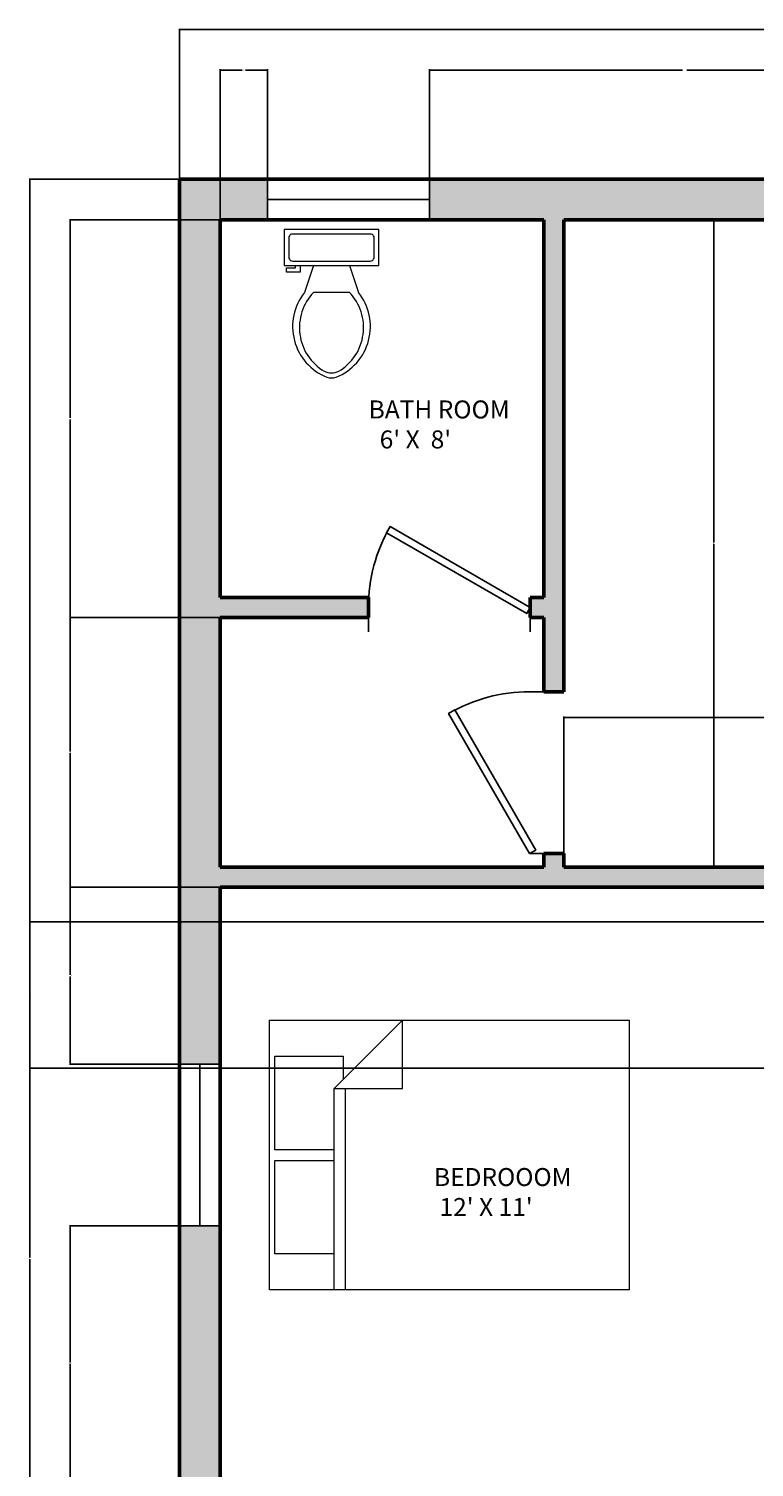
# Model space of a CAD drawing. Units: inches. Extents: x 4 to 671, y -79 to 570.
# Tile 3 of 7: x 4 to 165, y 250 to 570. Entities that reach past the tile are written whole.
import ezdxf

# ---------------------------------------------------------------- set-up
doc = ezdxf.new("R2010")
doc.units = ezdxf.units.IN
doc.header["$MEASUREMENT"] = 0
for name, color, linetype, lineweight in [('A-ANNO-DIMS', 2, 'Continuous', 18), ('A-AREA-IDEN', 7, 'Continuous', 18), ('A-WALL', 7, 'Continuous', 50), ('A-WALL-PATT', 251, 'Continuous', 13), ('bathroom', 90, 'Continuous', 18), ('doors', 40, 'Continuous', 25), ('furniture', 220, 'Continuous', 18), ('window', 30, 'Continuous', 25)]:
    doc.layers.add(name, color=color, linetype=linetype, lineweight=lineweight)
doc.styles.get("Standard").update_dxf_attribs({"font": 'arial.ttf'})
doc.dimstyles.get("Standard").update_dxf_attribs({"dimtxt": 0.18, "dimasz": 0.18, "dimexe": 0.18, "dimexo": 0.0625, "dimgap": 0.09, "dimtad": 0, "dimtih": 1, "dimtoh": 1, "dimdec": 4, "dimzin": 0, "dimdsep": 46, "dimtxsty": 'Standard', "dimcen": 0.09, "dimadec": 0, "dimazin": 0, "dimtfac": 1, "dimtdec": 4, "dimtofl": 0, "dimtmove": 0, "dimatfit": 3, "dimfxl": 1, "dimtolj": 1, "dimtzin": 0, "dimarcsym": 0})

# ---------------------------------------------------------------- blocks, each defined once
blk = doc.blocks.new('*U9')
for p, q in [((0, 0), (0, -6)), ((40, 0), (40, -6))]:
    blk.add_line(p, q)
blk.add_lwpolyline([(0, 0), (34.64, 20), (35.52, 18.48), (0.87, -1.52)], close=True)
blk.add_arc((0, 0), 40, 0, 30)
blk = doc.blocks.new('*U11')
for p, q in [((0, 0), (0, 6)), ((40, 0), (40, 6))]:
    blk.add_line(p, q)
blk.add_lwpolyline([(0, 0), (34.64, -20), (35.52, -18.48), (0.87, 1.52)], close=True)
blk.add_arc((0, 0), 40, 330, 0)
blk = doc.blocks.new('Bed - Queen')
for p, q in [((0, -80.00003), (0, 0)), ((0, 0), (59.99999, 0)), ((59.99999, 0), (59.99999, -80.00003)), ((7.99999, -1.2), (28.79998, -1.2)), ((7.99999, -14.4), (7.99999, -1.2)), ((28.79998, -1.2), (28.79998, -14.4)), ((31.19999, -1.2), (51.99999, -1.2)), ((31.19999, -14.4), (31.19999, -1.2)), ((51.99999, -1.2), (51.99999, -16.4)), ((0, -14.4), (44.8, -14.4)), ((59.99999, -29.6), (44.8, -14.4)), ((44.8, -14.4), (44.8, -29.6)), ((44.8, -16.8), (0, -16.8)), ((51.99999, -16.4), (46.79936, -16.4)), ((44.8, -29.6), (59.99999, -29.6)), ((59.99999, -80.00003), (0, -80.00003))]:
    blk.add_line(p, q)
blk = doc.blocks.new('Toilet - top')
for p, q in [((9.5, -6), (9.5, -2)), ((-10, -8.5), (-8, -8.5)), ((-10, -9.5), (-10, -8.5)), ((-7, -9.5), (-10, -9.5)), ((-8, -8.5), (-8, -8)), ((-7, -8), (-7, -9.5)), ((-4, -8), (-6, -14)), ((4, -8), (6, -14)), ((4, -14), (-4, -14))]:
    blk.add_line(p, q)
blk.add_lwpolyline([(10.5, -8), (10.5, 0), (-10.5, 0), (-10.5, -8)], close=True)
for points in [[(-9.5, -2), (-9.5, -6)], [(8.5, -1), (-8.5, -1)], [(-8.5, -7), (8.5, -7)]]:
    blk.add_lwpolyline(points)
for centre, radius, start, end in [((-8.62, -1.88), 0.884, 81.8699, 188.1301), ((8.62, -1.88), 0.884, 351.8699, 98.1301), ((-8.62, -6.12), 0.884, 171.8699, 278.1301), ((8.62, -6.12), 0.884, 261.8699, 8.1301), ((3.52, -21.58), 12.17, 141.4691, 247.9714), ((4.2, -21.82), 11.33, 136.3677, 238.9468), ((-3.52, -21.58), 12.17, 292.0284, 38.5307), ((-4.2, -21.82), 11.33, 301.053, 43.6321), ((0, -27.88), 4, 245.7318, 294.2682), ((0, -29), 4, 254.8605, 285.1395)]:
    blk.add_arc(centre, radius, start, end)
blk = doc.blocks.new('WIN-36')
for p, q in [((0, 0), (0, 9)), ((0, 9), (36, 9)), ((36, 9), (36, 0)), ((36, 9), (36, 4.5)), ((36, 4.5), (0, 4.5)), ((36, 0), (0, 0))]:
    blk.add_line(p, q)
blk = doc.blocks.new('*D49')
at = {"layer": 'A-ANNO-DIMS', "color": 0, "lineweight": -2, "transparency": 16777216}
for p, q in [((37.44, 536.41), (37.44, 569.83)), ((37.62, 569.65), (337.15, 569.65)), ((637.26, 569.65), (337.73, 569.65)), ((637.44, 536.41), (637.44, 569.83))]:
    blk.add_line(p, q, dxfattribs=at)
at = {"layer": 'A-ANNO-DIMS', "color": 0, "transparency": 16777216}
for points in [[(37.62, 569.68), (37.62, 569.62), (37.44, 569.65)], [(637.26, 569.68), (637.26, 569.62), (637.44, 569.65)]]:
    blk.add_solid(points, dxfattribs=at)
at = {"layer": 'Defpoints', "color": 0, "transparency": 16777216}
for p in [(637.44, 569.65), (37.44, 536.35), (637.44, 536.35)]:
    blk.add_point(p, dxfattribs=at)
at = {"layer": 'A-ANNO-DIMS', "color": 0, "transparency": 16777216, "insert": (337.44, 569.65), "char_height": 0.18, "attachment_point": 5}
blk.add_mtext('\\A1;600', dxfattribs=at)
blk = doc.blocks.new('*D51')
at = {"layer": 'A-ANNO-DIMS', "color": 0, "lineweight": -2, "transparency": 16777216}
for p, q in [((37.38, 536.35), (3.96, 536.35)), ((4.14, 536.17), (4.14, 296.53)), ((4.14, 56.53), (4.14, 296.17)), ((37.38, 56.35), (3.96, 56.35))]:
    blk.add_line(p, q, dxfattribs=at)
at = {"layer": 'A-ANNO-DIMS', "color": 0, "transparency": 16777216}
for points in [[(4.11, 536.17), (4.17, 536.17), (4.14, 536.35)], [(4.11, 56.53), (4.17, 56.53), (4.14, 56.35)]]:
    blk.add_solid(points, dxfattribs=at)
at = {"layer": 'Defpoints', "color": 0, "transparency": 16777216}
for p in [(4.14, 536.35), (37.44, 536.35), (37.44, 56.35)]:
    blk.add_point(p, dxfattribs=at)
at = {"layer": 'A-ANNO-DIMS', "color": 0, "transparency": 16777216, "insert": (4.14, 296.35), "char_height": 0.18, "attachment_point": 5}
blk.add_mtext('\\A1;480', dxfattribs=at)
blk = doc.blocks.new('*D59')
at = {"layer": 'A-ANNO-DIMS', "color": 0, "lineweight": -2, "transparency": 16777216}
for p, q in [((122.94, 383.41), (122.94, 416.83)), ((123.12, 416.65), (206.66, 416.65)), ((290.76, 416.65), (207.22, 416.65)), ((290.94, 383.41), (290.94, 416.83))]:
    blk.add_line(p, q, dxfattribs=at)
at = {"layer": 'A-ANNO-DIMS', "color": 0, "transparency": 16777216}
for points in [[(123.12, 416.68), (123.12, 416.62), (122.94, 416.65)], [(290.76, 416.68), (290.76, 416.62), (290.94, 416.65)]]:
    blk.add_solid(points, dxfattribs=at)
at = {"layer": 'Defpoints', "color": 0, "transparency": 16777216}
for p in [(290.94, 416.65), (122.94, 383.35), (290.94, 383.35)]:
    blk.add_point(p, dxfattribs=at)
at = {"layer": 'A-ANNO-DIMS', "color": 0, "transparency": 16777216, "insert": (206.94, 416.65), "char_height": 0.18, "attachment_point": 5}
blk.add_mtext('\\A1;168', dxfattribs=at)
blk = doc.blocks.new('*D60')
at = {"layer": 'A-ANNO-DIMS', "color": 0, "lineweight": -2, "transparency": 16777216}
for p, q in [((123, 527.35), (156.42, 527.35)), ((156.24, 527.17), (156.24, 455.53)), ((156.24, 383.53), (156.24, 455.17)), ((123, 383.35), (156.42, 383.35))]:
    blk.add_line(p, q, dxfattribs=at)
at = {"layer": 'A-ANNO-DIMS', "color": 0, "transparency": 16777216}
for points in [[(156.21, 527.17), (156.27, 527.17), (156.24, 527.35)], [(156.21, 383.53), (156.27, 383.53), (156.24, 383.35)]]:
    blk.add_solid(points, dxfattribs=at)
at = {"layer": 'Defpoints', "color": 0, "transparency": 16777216}
for p in [(122.94, 527.35), (122.94, 383.35), (156.24, 383.35)]:
    blk.add_point(p, dxfattribs=at)
at = {"layer": 'A-ANNO-DIMS', "color": 0, "transparency": 16777216, "insert": (156.24, 455.35), "char_height": 0.18, "attachment_point": 5}
blk.add_mtext('\\A1;144', dxfattribs=at)
blk = doc.blocks.new('*D69')
at = {"layer": 'A-ANNO-DIMS', "color": 0, "lineweight": -2, "transparency": 16777216}
for p, q in [((46.38, 303.54), (12.96, 303.54)), ((13.14, 303.36), (13.14, 273.13)), ((13.14, 242.53), (13.14, 272.76)), ((46.38, 242.35), (12.96, 242.35))]:
    blk.add_line(p, q, dxfattribs=at)
at = {"layer": 'A-ANNO-DIMS', "color": 0, "transparency": 16777216}
for points in [[(13.11, 303.36), (13.17, 303.36), (13.14, 303.54)], [(13.11, 242.53), (13.17, 242.53), (13.14, 242.35)]]:
    blk.add_solid(points, dxfattribs=at)
at = {"layer": 'Defpoints', "color": 0, "transparency": 16777216}
for p in [(13.14, 303.54), (46.44, 303.54), (46.44, 242.35)]:
    blk.add_point(p, dxfattribs=at)
at = {"layer": 'A-ANNO-DIMS', "color": 0, "transparency": 16777216, "insert": (13.14, 272.94), "char_height": 0.18, "attachment_point": 5}
blk.add_mtext('\\A1;61.19', dxfattribs=at)
blk = doc.blocks.new('*D70')
at = {"layer": 'A-ANNO-DIMS', "color": 0, "lineweight": -2, "transparency": 16777216}
for p, q in [((46.38, 378.85), (12.96, 378.85)), ((13.14, 378.67), (13.14, 359.38)), ((13.14, 339.72), (13.14, 359.01)), ((46.38, 339.54), (12.96, 339.54))]:
    blk.add_line(p, q, dxfattribs=at)
at = {"layer": 'A-ANNO-DIMS', "color": 0, "transparency": 16777216}
for points in [[(13.11, 378.67), (13.17, 378.67), (13.14, 378.85)], [(13.11, 339.72), (13.17, 339.72), (13.14, 339.54)]]:
    blk.add_solid(points, dxfattribs=at)
at = {"layer": 'Defpoints', "color": 0, "transparency": 16777216}
for p in [(13.14, 378.85), (46.44, 378.85), (46.44, 339.54)]:
    blk.add_point(p, dxfattribs=at)
at = {"layer": 'A-ANNO-DIMS', "color": 0, "transparency": 16777216, "insert": (13.14, 359.19), "char_height": 0.18, "attachment_point": 5}
blk.add_mtext('\\A1;39.314', dxfattribs=at)
blk = doc.blocks.new('*D71')
at = {"layer": 'A-ANNO-DIMS', "color": 0, "lineweight": -2, "transparency": 16777216}
for p, q in [((46.38, 438.85), (12.96, 438.85)), ((13.14, 438.67), (13.14, 409.03)), ((13.14, 379.03), (13.14, 408.67)), ((46.38, 378.85), (12.96, 378.85))]:
    blk.add_line(p, q, dxfattribs=at)
at = {"layer": 'A-ANNO-DIMS', "color": 0, "transparency": 16777216}
for points in [[(13.11, 438.67), (13.17, 438.67), (13.14, 438.85)], [(13.11, 379.03), (13.17, 379.03), (13.14, 378.85)]]:
    blk.add_solid(points, dxfattribs=at)
at = {"layer": 'Defpoints', "color": 0, "transparency": 16777216}
for p in [(13.14, 438.85), (46.44, 438.85), (46.44, 378.85)]:
    blk.add_point(p, dxfattribs=at)
at = {"layer": 'A-ANNO-DIMS', "color": 0, "transparency": 16777216, "insert": (13.14, 408.85), "char_height": 0.18, "attachment_point": 5}
blk.add_mtext('\\A1;60', dxfattribs=at)
blk = doc.blocks.new('*D72')
at = {"layer": 'A-ANNO-DIMS', "color": 0, "lineweight": -2, "transparency": 16777216}
for p, q in [((46.38, 527.35), (12.96, 527.35)), ((13.14, 527.17), (13.14, 483.28)), ((13.14, 439.03), (13.14, 482.92)), ((46.38, 438.85), (12.96, 438.85))]:
    blk.add_line(p, q, dxfattribs=at)
at = {"layer": 'A-ANNO-DIMS', "color": 0, "transparency": 16777216}
for points in [[(13.11, 527.17), (13.17, 527.17), (13.14, 527.35)], [(13.11, 439.03), (13.17, 439.03), (13.14, 438.85)]]:
    blk.add_solid(points, dxfattribs=at)
at = {"layer": 'Defpoints', "color": 0, "transparency": 16777216}
for p in [(13.14, 527.35), (46.44, 527.35), (46.44, 438.85)]:
    blk.add_point(p, dxfattribs=at)
at = {"layer": 'A-ANNO-DIMS', "color": 0, "transparency": 16777216, "insert": (13.14, 483.1), "char_height": 0.18, "attachment_point": 5}
blk.add_mtext('\\A1;88.5', dxfattribs=at)
blk = doc.blocks.new('*D80')
at = {"layer": 'A-ANNO-DIMS', "color": 0, "lineweight": -2, "transparency": 16777216}
for p, q in [((46.44, 527.41), (46.44, 560.83)), ((46.62, 560.65), (51.34, 560.65)), ((56.83, 560.65), (52.11, 560.65)), ((57.01, 527.41), (57.01, 560.83))]:
    blk.add_line(p, q, dxfattribs=at)
at = {"layer": 'A-ANNO-DIMS', "color": 0, "transparency": 16777216}
for points in [[(46.62, 560.68), (46.62, 560.62), (46.44, 560.65)], [(56.83, 560.68), (56.83, 560.62), (57.01, 560.65)]]:
    blk.add_solid(points, dxfattribs=at)
at = {"layer": 'Defpoints', "color": 0, "transparency": 16777216}
for p in [(57.01, 560.65), (46.44, 527.35), (57.01, 527.35)]:
    blk.add_point(p, dxfattribs=at)
at = {"layer": 'A-ANNO-DIMS', "color": 0, "transparency": 16777216, "insert": (51.72, 560.65), "char_height": 0.18, "attachment_point": 5}
blk.add_mtext('\\A1;10.57', dxfattribs=at)
blk = doc.blocks.new('*D81')
at = {"layer": 'A-ANNO-DIMS', "color": 0, "lineweight": -2, "transparency": 16777216}
for p, q in [((93.01, 527.41), (93.01, 560.83)), ((93.19, 560.65), (149.33, 560.65)), ((206.38, 560.65), (150.24, 560.65)), ((206.56, 527.41), (206.56, 560.83))]:
    blk.add_line(p, q, dxfattribs=at)
at = {"layer": 'A-ANNO-DIMS', "color": 0, "transparency": 16777216}
for points in [[(93.19, 560.68), (93.19, 560.62), (93.01, 560.65)], [(206.38, 560.68), (206.38, 560.62), (206.56, 560.65)]]:
    blk.add_solid(points, dxfattribs=at)
at = {"layer": 'Defpoints', "color": 0, "transparency": 16777216}
for p in [(206.56, 560.65), (93.01, 527.35), (206.56, 527.35)]:
    blk.add_point(p, dxfattribs=at)
at = {"layer": 'A-ANNO-DIMS', "color": 0, "transparency": 16777216, "insert": (149.79, 560.65), "char_height": 0.18, "attachment_point": 5}
blk.add_mtext('\\A1;113.55', dxfattribs=at)
blk = doc.blocks.new('*D94')
at = {"layer": 'A-ANNO-DIMS', "color": 0, "lineweight": -2, "transparency": 16777216}
for p, q in [((515.23, 371.2), (3.96, 371.2)), ((4.14, 371.02), (4.14, 355.08)), ((4.14, 338.78), (4.14, 354.72)), ((515.23, 338.6), (3.96, 338.6))]:
    blk.add_line(p, q, dxfattribs=at)
at = {"layer": 'A-ANNO-DIMS', "color": 0, "transparency": 16777216}
for points in [[(4.11, 371.02), (4.17, 371.02), (4.14, 371.2)], [(4.11, 338.78), (4.17, 338.78), (4.14, 338.6)]]:
    blk.add_solid(points, dxfattribs=at)
at = {"layer": 'Defpoints', "color": 0, "transparency": 16777216}
for p in [(4.14, 371.2), (515.3, 371.2), (515.3, 338.6)]:
    blk.add_point(p, dxfattribs=at)
at = {"layer": 'A-ANNO-DIMS', "color": 0, "transparency": 16777216, "insert": (4.14, 354.9), "char_height": 0.18, "attachment_point": 5}
blk.add_mtext('\\A1;32.6', dxfattribs=at)

msp = doc.modelspace()

# ---------------------------------------------------------------- hatches: boundary and pattern name
at = {"layer": 'A-WALL-PATT'}
h = msp.add_hatch(color=256, dxfattribs=at)
h.dxf.hatch_style = 1
h.paths.add_polyline_path([(46.4392, 165.2664), (37.4392, 165.2664), (37.4392, 108.5522), (41.9392, 108.5522), (46.4392, 108.5522), (46.4392, 117.8513), (151.434, 117.8513), (151.434, 120.1013), (151.434, 122.3513), (46.4392, 122.3513)], flags=17)
h.paths.add_polyline_path([(194.9392, 203.3513), (190.4392, 203.3513), (190.4392, 122.3513), (187.434, 122.3513), (187.434, 117.8513), (190.4392, 117.8513), (190.4392, 65.3513), (46.4392, 65.3513), (46.4392, 72.5522), (37.4392, 72.5522), (37.4392, 56.3513), (218.8007, 56.3513), (218.8007, 65.3513), (194.9392, 65.3513)])
h.paths.add_polyline_path([(46.4392, 242.3513), (190.4392, 242.3513), (190.4392, 239.3513), (194.9392, 239.3513), (194.9392, 249.8513), (190.4392, 249.8513), (190.4392, 246.8513), (46.4392, 246.8513), (46.4392, 303.5372), (37.4392, 303.5372), (37.4392, 201.2664), (41.9392, 201.2664), (46.4392, 201.2664)])
h.paths.add_polyline_path([(46.4392, 378.8513), (190.4392, 378.8513), (190.4392, 285.8513), (194.9392, 285.8513), (194.9392, 378.8513), (295.4392, 378.8513), (295.4392, 386.3513), (290.9392, 386.3513), (290.9392, 383.3513), (122.9392, 383.3513), (122.9392, 386.3513), (118.4392, 386.3513), (118.4392, 383.3513), (46.4392, 383.3513), (46.4392, 438.8513), (79.4392, 438.8513), (79.4392, 443.3513), (46.4392, 443.3513), (46.4392, 527.3513), (57.0095, 527.3513), (57.0095, 536.3513), (37.4392, 536.3513), (37.4392, 339.5372), (41.9392, 339.5372), (46.4392, 339.5372)])
h = msp.add_hatch(color=256, dxfattribs=at)
h.dxf.hatch_style = 1
h.paths.add_polyline_path([(206.5642, 536.3513), (93.0095, 536.3513), (93.0095, 531.8513), (93.0095, 527.3513), (118.4392, 527.3513), (118.4392, 443.3513), (115.4392, 443.3513), (115.4392, 438.8513), (118.4392, 438.8513), (118.4392, 422.3513), (120.6892, 422.3513), (122.9392, 422.3513), (122.9392, 527.3513), (206.5642, 527.3513)])
h.paths.add_polyline_path([(305.1113, 536.3513), (242.5642, 536.3513), (242.5642, 531.8513), (242.5642, 527.3513), (290.9392, 527.3513), (290.9392, 422.3513), (293.1892, 422.3513), (295.4392, 422.3513), (295.4392, 438.8513), (301.4392, 438.8513), (301.4392, 443.3513), (295.4392, 443.3513), (295.4392, 527.3513), (305.1113, 527.3513)])
h.paths.add_polyline_path([(454.1293, 536.3513), (341.1113, 536.3513), (341.1113, 531.8513), (341.1113, 527.3513), (355.4392, 527.3513), (355.4392, 443.3513), (325.4392, 443.3513), (325.4392, 438.8513), (355.4392, 438.8513), (355.4392, 422.3513), (359.9392, 422.3513), (359.9392, 527.3513), (454.1293, 527.3513)])
h.paths.add_polyline_path([(637.4392, 536.3513), (490.1293, 536.3513), (490.1293, 531.8513), (490.1293, 527.3513), (527.9392, 527.3513), (527.9392, 505.9443), (532.4392, 505.9443), (532.4392, 527.3513), (628.4392, 527.3513), (628.4392, 500.2662), (637.4392, 500.2662)])
h.paths.add_polyline_path([(637.4392, 464.2662), (628.4392, 464.2662), (628.4392, 383.3513), (556.4392, 383.3513), (532.4392, 383.3513), (532.4392, 469.9443), (527.9392, 469.9443), (527.9392, 383.3513), (359.9392, 383.3513), (359.9392, 386.3513), (355.4392, 386.3513), (355.4392, 378.8513), (403.4392, 378.8513), (403.4392, 318.8513), (407.9392, 318.8513), (407.9392, 378.8513), (551.9392, 378.8513), (551.9392, 290.3513), (554.1892, 290.3513, -0.01563646), (556.4392, 290.2809), (556.4392, 378.8513), (628.4392, 378.8513), (628.4392, 342.8513), (637.4392, 342.8513)])

# ---------------------------------------------------------------- linework, layer by layer
at = {"layer": 'A-WALL'}
for p, q in [((46.4392, 527.3513), (118.4392, 527.3513)), ((46.4392, 443.3513), (46.4392, 527.3513)), ((118.4392, 443.3513), (118.4392, 527.3513)), ((122.9392, 527.3513), (290.9392, 527.3513)), ((122.9392, 422.3513), (122.9392, 527.3513)), ((46.4392, 443.3513), (79.4392, 443.3513)), ((79.4392, 438.8513), (79.4392, 443.3513)), ((115.4392, 443.3513), (118.4392, 443.3513)), ((115.4392, 438.8513), (115.4392, 443.3513)), ((46.4392, 438.8513), (79.4392, 438.8513)), ((46.4392, 383.3513), (46.4392, 438.8513)), ((115.4392, 438.8513), (118.4392, 438.8513)), ((118.4392, 422.3513), (118.4392, 438.8513)), ((118.4392, 422.3513), (122.9392, 422.3513)), ((118.4392, 386.3513), (122.9392, 386.3513)), ((118.4392, 383.3513), (118.4392, 386.3513)), ((122.9392, 383.3513), (122.9392, 386.3513)), ((46.4392, 383.3513), (118.4392, 383.3513)), ((46.4392, 383.3513), (118.4392, 383.3513)), ((122.9392, 383.3513), (290.9392, 383.3513)), ((122.9392, 383.3513), (290.9392, 383.3513)), ((46.4392, 378.8513), (190.4392, 378.8513)), ((46.4392, 378.8513), (190.4392, 378.8513)), ((46.4392, 246.8513), (46.4392, 378.8513))]:
    msp.add_line(p, q, dxfattribs=at)
msp.add_lwpolyline([(313.4392, 56.3513), (37.4392, 56.3513), (37.4392, 536.3513), (637.4392, 536.3513), (637.4392, 56.3513), (362.9392, 56.3513)], dxfattribs=at)

# ---------------------------------------------------------------- block references
at = {"layer": 'bathroom'}
msp.add_blockref('Toilet - top', (71.2317, 525.1705), dxfattribs=at)
at = {"layer": 'doors', "xscale": 0.9, "yscale": 0.9, "zscale": 0.9}
for name, p, rotation in [('*U11', (115.4392, 441.1013), 180), ('*U9', (115.2892, 386.3513), 90)]:
    msp.add_blockref(name, p, dxfattribs=dict(at, rotation=rotation))
at = {"layer": 'furniture', "rotation": 90}
msp.add_blockref('Bed - Queen', (57.453, 289.2881), dxfattribs=at)
at = {"layer": 'window'}
msp.add_blockref('WIN-36', (57.0091, 527.351), dxfattribs=at)
at = {"layer": 'window', "rotation": 89.99999999999575}
msp.add_blockref('WIN-36', (46.4396, 303.5368), dxfattribs=at)

# ---------------------------------------------------------------- texts
at = {"layer": 'A-AREA-IDEN', "char_height": 4, "attachment_point": 1}
for s, insert in [("BATH ROOM\\P  6' X  8'", (79.5007, 487.1491)), ("BEDROOOM\\P 12' X 11'", (94.0298, 316.4002))]:
    msp.add_mtext_dynamic_manual_height_columns(s, width=44.806469, gutter_width=1, heights=[0], dxfattribs=dict(at, insert=insert))

# ---------------------------------------------------------------- dimensions: what is measured, and where the dimension line sits
at = {"layer": 'A-ANNO-DIMS'}
for base, p1, p2, override, picture, middle in [((637.4392, 569.6513), (37.4392, 536.3513), (637.4392, 536.3513), {"dimdec": 0, "dimlfac": 1, "dimrnd": 0, "dimzin": 0, "dimdsep": 46, "dimlunit": 2}, '*D49', (337.4392, 569.6513)), ((57.0095, 560.6513), (46.4392, 527.3513), (57.0095, 527.3513), {"dimdec": 2, "dimlfac": 1, "dimrnd": 0, "dimzin": 0, "dimdsep": 46, "dimlunit": 2}, '*D80', (51.7244, 560.6513)), ((206.5642, 560.6513), (93.0095, 527.3513), (206.5642, 527.3513), {"dimdec": 2, "dimlfac": 1, "dimrnd": 0, "dimzin": 0, "dimdsep": 46, "dimlunit": 2}, '*D81', (149.7868, 560.6513)), ((290.9392, 416.6513), (122.9392, 383.3513), (290.9392, 383.3513), {"dimdec": 0, "dimlfac": 1, "dimrnd": 0, "dimzin": 0, "dimdsep": 46, "dimlunit": 2}, '*D59', (206.9392, 416.6513))]:
    dim = msp.add_linear_dim(base=base, p1=p1, p2=p2, dimstyle='Standard', override=override, dxfattribs=at)
    dim.commit()
    dim.dimension.update_dxf_attribs({"geometry": picture, "text_midpoint": middle})
for base, p1, p2, angle, override, picture, middle in [((4.1392, 536.3513), (37.4392, 56.3513), (37.4392, 536.3513), 90, {"dimdec": 0, "dimlfac": 1, "dimrnd": 0, "dimzin": 0, "dimdsep": 46, "dimlunit": 2}, '*D51', (4.1392, 296.3513)), ((13.1392, 527.3513), (46.4392, 438.8513), (46.4392, 527.3513), 90, {"dimdec": 1, "dimlfac": 1, "dimrnd": 0, "dimzin": 0, "dimdsep": 46, "dimlunit": 2}, '*D72', (13.1392, 483.1013)), ((156.2392, 383.3513), (122.9392, 527.3513), (122.9392, 383.3513), 270, {"dimdec": 0, "dimlfac": 1, "dimrnd": 0, "dimzin": 0, "dimdsep": 46, "dimlunit": 2}, '*D60', (156.2392, 455.3513)), ((13.1392, 438.8513), (46.4392, 378.8513), (46.4392, 438.8513), 90, {"dimdec": 0, "dimlfac": 1, "dimrnd": 0, "dimzin": 0, "dimdsep": 46, "dimlunit": 2}, '*D71', (13.1392, 408.8513)), ((13.1392, 378.8513), (46.4392, 339.5372), (46.4392, 378.8513), 90, {"dimdec": 3, "dimlfac": 1, "dimrnd": 0, "dimzin": 0, "dimdsep": 46, "dimlunit": 2}, '*D70', (13.1392, 359.1942)), ((4.1392, 371.2019), (515.2973, 338.599), (515.2973, 371.2019), 90, {"dimdec": 1, "dimlfac": 1, "dimrnd": 0, "dimzin": 0, "dimdsep": 46, "dimlunit": 2}, '*D94', (4.1392, 354.9005)), ((13.1392, 303.5372), (46.4392, 242.3513), (46.4392, 303.5372), 90, {"dimdec": 2, "dimlfac": 1, "dimrnd": 0, "dimzin": 0, "dimdsep": 46, "dimlunit": 2}, '*D69', (13.1392, 272.9442))]:
    dim = msp.add_linear_dim(base=base, p1=p1, p2=p2, angle=angle, dimstyle='Standard', override=override, dxfattribs=at)
    dim.commit()
    dim.dimension.update_dxf_attribs({"geometry": picture, "text_midpoint": middle})

doc.saveas('drawing.dxf')
